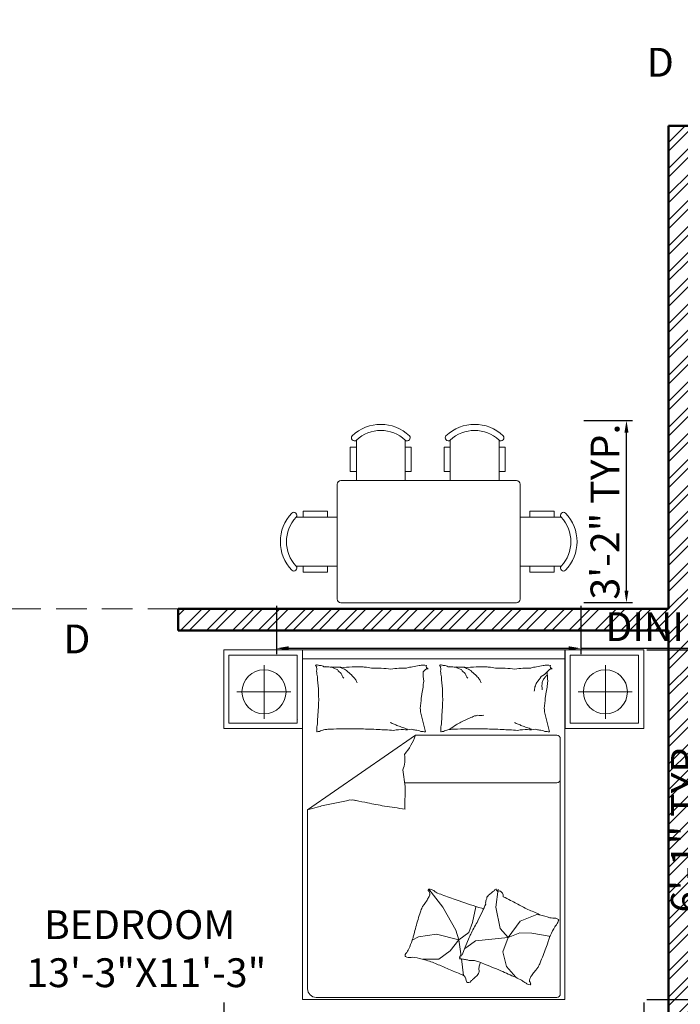
# Model space of a CAD drawing. Units: millimetres. Extents: x 67033 to 68301, y 155969 to 157209.
# Tile 12 of 17: x 67633 to 67771, y 156689 to 156894. Entities that reach past the tile are written whole.
import ezdxf

# ---------------------------------------------------------------- set-up
doc = ezdxf.new("R2010")
doc.units = ezdxf.units.MM
doc.linetypes.add('HIDDEN', pattern=[9.525, 6.35, -3.175])
for name, color, linetype, lineweight in [('A-ANNO-DIMS', 2, 'Continuous', 18), ('A-ANNO-TEXT', 7, 'Continuous', 18), ('A-AREA-IDEN', 3, 'Continuous', 18), ('A-FLOR-OVHD', 1, 'HIDDEN', 18), ('A-FLOR-PATT', 252, 'Continuous', 13), ('A-FURN', 8, 'Continuous', 18), ('A-WALL', 7, 'Continuous', 50), ('A-WALL-PATT', 8, 'Continuous', 13)]:
    doc.layers.add(name, color=color, linetype=linetype, lineweight=lineweight)
doc.styles.add('DIM_FONT', font='SIMPLEX.shx', dxfattribs={"width": 0.8})
doc.styles.get("Standard").update_dxf_attribs({"font": 'arial.ttf'})
doc.dimstyles.new('ISO-25', dxfattribs={"dimtxt": 6, "dimasz": 2.5, "dimexe": 1.25, "dimexo": 0.625, "dimtad": 1, "dimdec": 0, "dimlunit": 3, "dimtxsty": 'Standard', "dimcen": 2.5, "dimadec": 0, "dimazin": 0, "dimtfac": 1, "dimtdec": 0, "dimtmove": 0, "dimatfit": 3, "dimfxl": 1, "dimarcsym": 0})

# ---------------------------------------------------------------- blocks, each defined once
blk = doc.blocks.new('A$C79766A75')
for p, q in [((0.45, 1.9999), (0, 1.9999)), ((0, 1.9999), (0, 1.5499)), ((0.45, 1.5499), (0.45, 1.9999)), ((1.9506, 2), (0.4506, 2)), ((0.4506, 2), (0.4506, 0)), ((1.9506, 0), (1.9506, 2)), ((2.402, 1.9999), (1.952, 1.9999)), ((1.952, 1.9999), (1.952, 1.5499)), ((2.402, 1.5499), (2.402, 1.9999)), ((0.42, 1.9699), (0.03, 1.9699)), ((0.03, 1.9699), (0.03, 1.5799)), ((0.42, 1.5799), (0.42, 1.9699)), ((1.9506, 1.9476), (0.4506, 1.9476)), ((2.372, 1.9699), (1.982, 1.9699)), ((1.982, 1.9699), (1.982, 1.5799)), ((2.372, 1.5799), (2.372, 1.9699)), ((0.2304, 1.9125), (0.2304, 1.6061)), ((2.1824, 1.9125), (2.1824, 1.6061)), ((0.0743, 1.7595), (0.3834, 1.7595)), ((2.0263, 1.7595), (2.3354, 1.7595)), ((1.1461, 1.5617), (1.1254, 1.6443)), ((1.8553, 1.5617), (1.8346, 1.6443)), ((0.03, 1.5799), (0.42, 1.5799)), ((0.4234, 1.6034), (0.4228, 1.6034)), ((1.982, 1.5799), (2.372, 1.5799)), ((0, 1.5499), (0.45, 1.5499)), ((1.1536, 1.5317), (1.1461, 1.5617)), ((1.8628, 1.5317), (1.8553, 1.5617)), ((1.952, 1.5499), (2.402, 1.5499)), ((1.0972, 1.5115), (0.4791, 1.0841)), ((1.0972, 1.5115), (1.9048, 1.5115)), ((1.9248, 1.4915), (1.9248, 0.0322)), ((1.0383, 1.2184), (1.0246, 1.3138)), ((1.9048, 1.2389), (1.0354, 1.2389)), ((1.0365, 1.0883), (1.0383, 1.2184)), ((0.4791, 0.0622), (0.4791, 1.0841)), ((1.1731, 0.6316), (1.2523, 0.5276)), ((1.5696, 0.6317), (1.5559, 0.5286)), ((1.2523, 0.5276), (1.3274, 0.3973)), ((1.4223, 0.4407), (1.442, 0.5296)), ((1.5559, 0.5286), (1.5817, 0.4065)), ((1.6952, 0.4478), (1.7898, 0.4856)), ((1.7898, 0.4856), (1.8139, 0.4822)), ((1.3274, 0.3973), (1.3452, 0.342)), ((1.4025, 0.3834), (1.4223, 0.4407)), ((1.5817, 0.4065), (1.6264, 0.355)), ((1.6264, 0.355), (1.6952, 0.4478)), ((1.1139, 0.3597), (1.0779, 0.3397)), ((1.2167, 0.3736), (1.1139, 0.3597)), ((1.3452, 0.342), (1.2167, 0.3736)), ((1.2957, 0.2787), (1.3452, 0.342)), ((1.3452, 0.342), (1.4025, 0.3834)), ((1.3452, 0.342), (1.3569, 0.2478)), ((1.4034, 0.3558), (1.3803, 0.2995)), ((1.6264, 0.355), (1.4406, 0.3361)), ((1.5954, 0.2725), (1.6264, 0.355)), ((1.6264, 0.355), (1.6935, 0.3825)), ((1.6935, 0.3825), (1.7623, 0.379)), ((1.7623, 0.379), (1.8603, 0.3619)), ((1.8603, 0.3619), (1.8636, 0.3554)), ((1.3803, 0.2995), (1.3626, 0.256)), ((1.3907, 0.3), (1.3787, 0.2914)), ((1.4406, 0.3361), (1.3907, 0.3)), ((1.1376, 0.2313), (1.2305, 0.2313)), ((1.2305, 0.2313), (1.2957, 0.2787)), ((1.3588, 0.2331), (1.3706, 0.1385)), ((1.6161, 0.19), (1.5954, 0.2725)), ((1.6697, 0.1274), (1.6161, 0.19)), ((1.9048, 0.0122), (0.5291, 0.0122)), ((0.4506, 0), (1.9506, 0))]:
    blk.add_line(p, q)
for centre in [(0.2304, 1.7595), (2.1824, 1.7595)]:
    blk.add_circle(centre, 0.126)
for centre, radius, start, end in [((0.5246, 1.9378), 0.0251, 274.3025, 291.7883), ((0.5486, 1.9393), 0.0289, 239.3487, 274.3025), ((1.2338, 1.9378), 0.0251, 274.3025, 291.7883), ((1.2578, 1.9393), 0.0289, 239.3487, 274.3025), ((0.5232, 1.9139), 0.00342, 291.7883, 340.436), ((0.525, 1.9085), 0.00232, 340.436, 101.8931), ((0.5311, 1.9093), 0.00428, 201.9904, 281.8931), ((0.4996, 1.8889), 0.0328, 338.579, 8.1335), ((0.2896, 1.8253), 0.246, 8.1335, 12.1095), ((0.5465, 1.8994), 0.0156, 158.579, 201.9904), ((0.7297, 1.8867), 0.1983, 187.6809, 192.1095), ((0.5458, 1.8568), 0.0539, 59.3487, 84.7408), ((0.546, 1.0829), 0.8208, 84.7408, 88.0921), ((0.6118, 2.0005), 0.0992, 254.0648, 274.2159), ((0.6775, 1.9817), 0.0992, 233.9136, 254.0648), ((0.6362, 0.406), 1.4943, 88.0921, 90.5757), ((0.7304, 1.9449), 0.0992, 216.1766, 233.9136), ((0.7737, 2.1075), 0.234, 242.7604, 249.1397), ((0.7661, 1.8961), 0.0992, 198.4397, 216.1766), ((0.7591, 1.0293), 0.8732, 90.5757, 94.8018), ((0.738, 1.949), 0.0768, 231.6114, 242.7604), ((0.974, 2.1633), 0.3916, 226.1885, 231.6114), ((0.7631, 2.1919), 0.2897, 267.4614, 274.8018), ((0.8143, 2.0532), 0.1524, 259.8101, 267.4614), ((0.7515, 1.3747), 0.5293, 79.8101, 83.9133), ((0.8451, 0.8466), 1.049, 83.9133, 90), ((1.046, 1.2129), 0.6827, 90, 97.5469), ((1.1117, 1.6625), 0.2422, 97.5469, 105.744), ((1.0352, 2.2041), 0.3048, 278.4372, 285.744), ((1.1179, 2.0719), 0.1611, 270, 278.4372), ((1.171, 1.8579), 0.0342, 94.4002, 153.4195), ((1.6324, 1.8735), 0.4918, 180, 186.2324), ((1.1592, 2.0011), 0.0904, 258.7276, 270), ((1.1709, 1.9049), 0.0131, 153.4195, 258.7276), ((1.2325, 1.9139), 0.00342, 291.7883, 340.436), ((1.2342, 1.9085), 0.00232, 340.436, 101.8931), ((1.2404, 1.9093), 0.00428, 201.9904, 281.8931), ((1.2088, 1.8889), 0.0328, 338.579, 8.1335), ((0.9988, 1.8253), 0.246, 8.1335, 12.1095), ((1.2558, 1.8994), 0.0156, 158.579, 201.9904), ((1.4389, 1.8867), 0.1983, 187.6809, 192.1095), ((1.2551, 1.8568), 0.0539, 59.3487, 84.7408), ((1.2552, 1.0829), 0.8208, 84.7408, 88.0921), ((1.3211, 2.0005), 0.0992, 254.0648, 274.2159), ((1.3868, 1.9817), 0.0992, 233.9136, 254.0648), ((1.3455, 0.406), 1.4943, 88.0921, 90.5757), ((1.4396, 1.9449), 0.0992, 216.1766, 233.9136), ((1.4829, 2.1075), 0.234, 242.7604, 249.1397), ((1.4753, 1.8961), 0.0992, 198.4397, 216.1766), ((1.4683, 1.0293), 0.8732, 90.5757, 94.8018), ((1.4473, 1.949), 0.0768, 231.6114, 242.7604), ((1.6833, 2.1633), 0.3916, 226.1885, 231.6114), ((1.4724, 2.1919), 0.2897, 267.4614, 274.8018), ((1.5236, 2.0532), 0.1524, 259.8101, 267.4614), ((1.4607, 1.3747), 0.5293, 79.8101, 83.9133), ((1.5543, 0.8466), 1.049, 83.9133, 90), ((1.7552, 1.2129), 0.6827, 90, 97.5469), ((1.821, 1.6625), 0.2422, 97.5469, 105.744), ((1.7444, 2.2041), 0.3048, 278.4372, 285.744), ((1.7511, 1.9723), 0.1399, 297.2036, 314.9024), ((1.8271, 2.0719), 0.1611, 270, 278.4372), ((1.8802, 1.8579), 0.0342, 94.4002, 153.4195), ((2.3416, 1.8735), 0.4918, 180, 186.2324), ((1.8684, 2.0011), 0.0904, 258.7276, 270), ((1.8802, 1.9049), 0.0131, 153.4195, 258.7276), ((1.4472, 1.8987), 0.9131, 183.3687, 187.6809), ((0.9057, 1.9982), 0.2252, 219.0349, 226.1885), ((0.7932, 1.8591), 0.0493, 208.3168, 219.0349), ((0.9392, 1.9062), 0.2002, 203.0028, 208.3168), ((1.3446, 1.7858), 0.204, 170.3156, 180), ((2.1565, 1.8987), 0.9131, 183.3687, 187.6809), ((1.615, 1.9982), 0.2252, 219.0349, 226.1885), ((1.5025, 1.8591), 0.0493, 208.3168, 219.0349), ((1.6484, 1.9062), 0.2002, 203.0028, 208.3168), ((1.6554, 1.8529), 0.1399, 332.6012, 343.485), ((1.6908, 1.9123), 0.1399, 314.9024, 332.6012), ((1.7653, 1.8132), 0.0562, 341.2201, 0), ((1.6307, 1.8895), 0.2056, 338.1851, 341.2201), ((1.6887, 1.8881), 0.1511, 334.6449, 338.1851), ((1.7896, 1.8667), 0.0526, 318.5571, 334.6449), ((1.784, 1.9167), 0.0899, 306.2641, 318.5571), ((2.0538, 1.7858), 0.204, 170.3156, 180), ((1.2208, 1.7573), 0.6787, 178.3669, 183.3687), ((0.8192, 1.792), 0.3171, 347.8016, 351.9949), ((2.0027, 1.5994), 0.882, 167.8016, 170.3156), ((1.9301, 1.7573), 0.6787, 178.3669, 183.3687), ((1.6404, 1.8023), 0.1399, 343.485, 354.3689), ((1.73, 1.7719), 0.0915, 0, 14.6851), ((1.5284, 1.792), 0.3171, 347.8016, 351.9949), ((2.7119, 1.5994), 0.882, 167.8016, 170.3156), ((1.9066, 1.6447), 1.3652, 176.945, 178.3669), ((0.4711, 1.7556), 0.6588, 351.9949, 357.3351), ((2.6158, 1.6447), 1.3652, 176.945, 178.3669), ((1.1803, 1.7556), 0.6588, 351.9949, 357.3351), ((14.1519, 0.85), 13.6356, 176.49514, 176.94504), ((1.0578, 1.6474), 0.0677, 357.3351, 14.0452), ((14.8612, 0.85), 13.6356, 176.49514, 176.94504), ((1.767, 1.6474), 0.0677, 357.3351, 14.0452), ((0.8521, 1.5209), 0.3212, 170.0016, 176.4951), ((0.6583, 0.9067), 0.7387, 64.6889, 66.5156), ((1.5613, 1.5209), 0.3212, 170.0016, 176.4951), ((1.1895, 1.8508), 0.3126, 296.4985, 302.135), ((0.7658, 2.8912), 1.4323, 294.3265, 296.4985), ((1.226, 2.0834), 0.5066, 290.6743, 294.3265), ((1.4305, 1.6796), 0.058, 274.0828, 290.6743), ((1.4679, 1.8969), 0.2721, 266.4448, 274.0828), ((1.3675, 0.9067), 0.7387, 64.6889, 66.5156), ((0.513, 1.535), 0.0193, 350.0016, 16.6978), ((0.5322, 1.5304), 0.00132, 16.6978, 97.1204), ((0.5579, 1.4467), 0.0875, 97.1204, 106.2212), ((0.5822, 1.4654), 0.0767, 106.2212, 117.2841), ((0.5507, 1.5832), 0.0453, 282.869, 297.2841), ((0.5623, 1.6885), 0.1459, 273.574, 282.869), ((0.589, 2.7103), 1.164, 270.2865, 273.574), ((0.7584, 7.2662), 5.7185, 269.0296, 270.2865), ((0.9401, 4.9065), 3.3622, 267.3904, 269.0296), ((0.9811, 2.7573), 1.2165, 265.3824, 267.3904), ((0.8583, 0.139), 1.4048, 85.3824, 87.2509), ((1.0175, 1.3138), 0.2301, 87.2509, 101.5586), ((0.7015, 0.888), 0.7387, 66.5156, 68.3423), ((0.7501, 0.8688), 0.7387, 68.3423, 70.572), ((0.8043, 0.8497), 0.7387, 70.572, 72.8018), ((1.0449, 1.6886), 0.1459, 263.5659, 281.5586), ((1.1099, 1.6599), 0.1197, 252.6136, 263.5659), ((1.0587, 1.3144), 0.2297, 72.6136, 80.5159), ((1.108, 1.2635), 0.2708, 80.5159, 85.9171), ((1.1535, 1.5308), 0.000917, 85.9171, 194.0449), ((1.2222, 1.535), 0.0193, 350.0016, 16.6978), ((1.2414, 1.5304), 0.00132, 16.6978, 97.1204), ((1.2671, 1.4467), 0.0875, 97.1204, 106.2212), ((1.2914, 1.4654), 0.0767, 106.2212, 117.2841), ((1.2599, 1.5832), 0.0453, 282.869, 297.2841), ((1.2716, 1.6885), 0.1459, 273.574, 282.869), ((0.9025, 2.1618), 0.7286, 302.135, 305.8263), ((1.2982, 2.7103), 1.164, 270.2865, 273.574), ((1.4677, 7.2662), 5.7185, 269.0296, 270.2865), ((1.6493, 4.9065), 3.3622, 267.3904, 269.0296), ((1.6903, 2.7573), 1.2165, 265.3824, 267.3904), ((1.5676, 0.139), 1.4048, 85.3824, 87.2509), ((1.7268, 1.3138), 0.2301, 87.2509, 101.5586), ((1.4107, 0.888), 0.7387, 66.5156, 68.3423), ((1.4594, 0.8688), 0.7387, 68.3423, 70.572), ((1.5136, 0.8497), 0.7387, 70.572, 72.8018), ((1.7541, 1.6886), 0.1459, 263.5659, 281.5586), ((1.8192, 1.6599), 0.1197, 252.6136, 263.5659), ((1.7679, 1.3144), 0.2297, 72.6136, 80.5159), ((1.8172, 1.2635), 0.2708, 80.5159, 85.9171), ((1.8627, 1.5308), 0.000917, 85.9171, 194.0449), ((0.745, 1.6407), 0.3751, 320.3555, 339.8512), ((1.9048, 1.4915), 0.02, 0, 90), ((0.8556, 1.3759), 0.1801, 339.8512, 8.1356), ((1.9048, 1.2589), 0.02, 270, 0), ((-0.1888, 5.1029), 4.0646, 280.7276, 282.9255), ((0.7282, 1.1989), 0.0581, 262.2696, 280.7276), ((0.7833, 1.3309), 0.1942, 256.8096, 262.2696), ((0.2481, -1.3253), 2.5158, 76.8096, 78.3259), ((-0.0248, 2.8487), 1.8351, 285.9352, 287.7364), ((0.3872, 1.7415), 0.6574, 282.9255, 285.9352), ((0.3953, -1.4284), 2.588, 78.3259, 80.505), ((0.413, -2.64), 3.7801, 80.505, 82.308), ((1.1752, 0.6267), 0.0063, 166.7192, 233.4208), ((1.1734, 0.6272), 0.00443, 93.9484, 166.7192), ((1.163, 0.6103), 0.0142, 10.4074, 53.4208), ((1.1755, 0.5964), 0.0352, 69.6548, 93.9484), ((1.1669, 0.5731), 0.0601, 51.4146, 69.6548), ((1.2538, 0.682), 0.0792, 231.4146, 247.2931), ((1.1426, 1.1456), 0.6605, 306.2163, 307.2151), ((1.7751, 0.3162), 0.3825, 126.2163, 127.5287), ((1.5806, 0.5924), 0.0452, 127.5287, 134.1274), ((1.5093, 0.6825), 0.0697, 308.8136, 314.1274), ((1.5706, 0.6318), 0.0127, 176.7545, 308.8136), ((1.5621, 0.59), 0.0359, 356.7545, 62.7098), ((0.9961, 0.6678), 0.194, 320.2995, 329.0944), ((0.8605, 0.749), 0.352, 329.0944, 333.1821), ((1.1396, 0.6079), 0.0393, 333.1821, 345.4291), ((1.1011, 0.5989), 0.0771, 2.7286, 10.4074), ((1.1628, 0.6019), 0.0153, 345.4291, 2.7286), ((1.5463, 1.3811), 0.8371, 247.2931, 249.8713), ((3.0113, 5.3783), 5.0942, 249.8713, 250.9164), ((2.374, 3.5362), 3.145, 250.9164, 253.3915), ((1.5435, 0.5526), 0.0458, 157.5838, 188.0492), ((1.4828, 0.5833), 0.0226, 324.1064, 8.0492), ((1.4519, 0.6426), 0.0774, 313.5224, 324.1064), ((1.383, 0.7705), 0.2176, 307.2151, 313.5224), ((0.2201, -2.1858), 3.0972, 62.7098, 63.5853), ((2.5711, 2.3551), 2.0162, 242.5001, 243.5853), ((1.3115, 0.4414), 0.1965, 153.9265, 162.1604), ((1.2077, 0.4922), 0.081, 140.2995, 153.9265), ((1.5084, 0.6341), 0.1166, 253.3915, 259.2634), ((2.4089, 0.1204), 1.0054, 154.9471, 157.5838), ((4.5245, 5.9445), 6.1019, 242.15178, 242.50014), ((-0.9881, -4.647), 5.8383, 62.15178, 62.50792), ((1.5182, -0.068), 0.6236, 62.5079, 69.2514), ((3.0311, -0.112), 2.003, 162.1604, 164.7375), ((2.9813, -0.2643), 1.6868, 152.9116, 154.9471), ((1.7121, 0.0657), 0.43, 69.2514, 77.3748), ((1.8682, 0.4049), 0.063, 77.3748, 93.3881), ((1.8955, 0.5247), 0.0599, 256.9598, 273.3881), ((1.9257, 0.5082), 0.0509, 238.3083, 256.9598), ((1.9279, 0.441), 0.0168, 130.5086, 180.9614), ((1.9201, 0.4587), 0.0058, 180.9614, 238.3083), ((2.6887, -0.0186), 1.6481, 164.7375, 166.159), ((2.8096, -0.3311), 1.5652, 150.064, 152.9116), ((-0.5166, 1.5491), 2.6619, 333.6668, 334.8268), ((1.8435, 0.4743), 0.0755, 310.5086, 333.6668), ((-1.4109, 1.284), 2.6619, 338.0627, 339.2227), ((0.9098, 0.4035), 0.1798, 339.2227, 343.6878), ((0.5589, 0.5062), 0.5454, 343.6878, 346.159), ((1.2176, 0.4627), 0.2143, 330.064, 337.7645), ((1.3456, 0.5261), 0.5454, 339.2919, 341.7631), ((1.701, 0.4319), 0.1798, 334.8268, 339.2919), ((0.9882, 0.3177), 0.0755, 314.9045, 338.0627), ((3.6966, -0.4634), 2.003, 157.7645, 160.3416), ((3.4079, -0.2212), 1.6481, 160.3416, 161.7631), ((1.0533, 0.2524), 0.0168, 134.9045, 185.3572), ((1.0424, 0.2513), 0.0058, 185.3572, 242.7041), ((1.0631, 0.2914), 0.0509, 242.7041, 261.3557), ((1.0645, 0.3003), 0.0599, 261.3557, 277.784), ((1.0811, 0.1786), 0.063, 81.7707, 97.784), ((1.0286, -0.1846), 0.43, 73.6473, 81.7707), ((0.974, -0.3705), 0.6236, 66.9038, 73.6473), ((1.3465, 0.2383), 0.00467, 287.1867, 70.6201), ((1.3486, 0.2247), 0.0092, 70.6201, 94.2593), ((1.3694, 0.234), 0.0231, 107.1867, 157.7645), ((1.3563, 0.267), 0.034, 262.0178, 274.2593), ((1.4091, 0.4221), 0.1955, 255.1193, 262.0178), ((1.358, 0.0507), 0.1794, 75.1193, 82.3216), ((-1.0716, -5.1672), 5.8383, 66.54766, 66.9038), ((3.6805, 5.7866), 6.1019, 246.54766, 246.89602), ((2.0773, 2.0287), 2.0162, 246.896, 247.9812), ((1.4096, 0.153), 0.0712, 82.3216, 94.5118), ((1.4285, 0.2893), 0.0663, 261.8784, 274.5118), ((1.4755, 0.332), 0.1166, 248.9957, 261.8784), ((2.7121, 3.1012), 3.145, 246.5205, 248.9957), ((1.505, 0.1766), 0.0458, 161.9797, 192.4451), ((2.4175, -0.1202), 1.0054, 160.6552, 161.9797), ((1.6279, 0.2819), 0.194, 315.9036, 324.6985), ((1.856, 0.1288), 0.081, 135.9036, 149.5306), ((1.9797, 0.1108), 0.1965, 149.5306, 157.7645), ((0.1602, -2.7118), 3.0972, 67.1056, 67.9812), ((1.3512, 0.1084), 0.0359, 1.1504, 67.1056), ((1.6722, -0.1762), 0.3825, 130.6122, 131.9246), ((0.9933, 0.6156), 0.6605, 310.6122, 311.611), ((1.2874, 0.2845), 0.2176, 311.611, 317.9183), ((1.3914, 0.1905), 0.0774, 317.9183, 328.5023), ((1.4382, 0.1619), 0.0226, 328.5023, 12.4451), ((3.6993, 4.7998), 5.0942, 245.4754, 246.5205), ((2.051, 0.8725), 0.8371, 242.8972, 245.4754), ((1.7345, 0.1188), 0.0153, 341.0332, 358.3327), ((1.6723, 0.1058), 0.0771, 358.3327, 6.0115), ((1.7162, 0.1388), 0.0393, 328.7862, 341.0332), ((1.4661, 0.3294), 0.352, 324.6985, 328.7862), ((0.5291, 0.0622), 0.05, 180, 270), ((1.3997, 0.1094), 0.0127, 181.1504, 313.2095), ((1.3607, 0.1509), 0.0697, 313.2095, 318.5233), ((1.4468, 0.0748), 0.0452, 131.9246, 138.5233), ((1.7576, 0.1689), 0.0792, 227.0187, 242.8972), ((1.6963, 0.0438), 0.0601, 47.0187, 65.2589), ((1.737, 0.0526), 0.0352, 65.2589, 89.5525), ((1.7401, 0.0928), 0.0142, 6.0115, 49.0249), ((1.756, 0.0832), 0.00443, 89.5525, 162.3233), ((1.7602, 0.0924), 0.0063, 162.3233, 229.0249), ((1.9048, 0.0322), 0.02, 270, 0)]:
    blk.add_arc(centre, radius, start, end)
at = {"style": 'DIM_FONT', "text_generation_flag": 4, "width": 0.8, "flags": 9}
for tag in ['XSIZE', 'YSIZE']:
    blk.add_attdef(tag, (1.9506, 2), '', height=0.0005, rotation=180, dxfattribs=at)
blk = doc.blocks.new('table dining')
for p, q in [((67480.1, 156784.21), (67480.1, 156775.8)), ((67490.26, 156775.8), (67490.26, 156784.21)), ((67499.62, 156784.21), (67499.62, 156775.8)), ((67509.78, 156775.8), (67509.78, 156784.21)), ((67480.1, 156782.75), (67478.83, 156782.75)), ((67478.83, 156777.67), (67478.83, 156782.75)), ((67490.26, 156782.75), (67491.53, 156782.75)), ((67491.53, 156777.67), (67491.53, 156782.75)), ((67499.62, 156782.75), (67498.35, 156782.75)), ((67498.35, 156777.67), (67498.35, 156782.75)), ((67509.78, 156782.75), (67511.05, 156782.75)), ((67511.05, 156777.67), (67511.05, 156782.75)), ((67476.85, 156775.8), (67513.43, 156775.8)), ((67480.1, 156777.67), (67478.83, 156777.67)), ((67490.26, 156777.67), (67491.53, 156777.67)), ((67499.62, 156777.67), (67498.35, 156777.67)), ((67509.78, 156777.67), (67511.05, 156777.67)), ((67476.09, 156751.17), (67476.09, 156775.04)), ((67514.19, 156751.17), (67514.19, 156775.04)), ((67476.09, 156768.18), (67467.57, 156768.18)), ((67469.03, 156768.18), (67469.03, 156769.45)), ((67474.11, 156769.45), (67469.03, 156769.45)), ((67474.11, 156768.18), (67474.11, 156769.45)), ((67514.19, 156768.18), (67522.71, 156768.18)), ((67516.16, 156768.18), (67516.16, 156769.45)), ((67516.16, 156769.45), (67521.24, 156769.45)), ((67521.24, 156768.18), (67521.24, 156769.45)), ((67467.57, 156758.02), (67476.09, 156758.02)), ((67469.03, 156758.02), (67469.03, 156756.75)), ((67474.11, 156758.02), (67474.11, 156756.75)), ((67522.71, 156758.02), (67514.19, 156758.02)), ((67516.16, 156758.02), (67516.16, 156756.75)), ((67521.24, 156758.02), (67521.24, 156756.75)), ((67474.11, 156756.75), (67469.03, 156756.75)), ((67516.16, 156756.75), (67521.24, 156756.75)), ((67476.85, 156750.4), (67513.43, 156750.4))]:
    blk.add_line(p, q)
for centre, radius, start, end in [((67485.18, 156778.87), 8.64, 46.4394, 133.5606), ((67485.18, 156778.87), 7.37, 46.4394, 133.5606), ((67504.7, 156778.87), 8.64, 46.4394, 133.5606), ((67504.7, 156778.87), 7.37, 46.4394, 133.5606), ((67479.7, 156784.71), 0.637, 138.3417, 308.7795), ((67490.66, 156784.71), 0.637, 231.2205, 41.6583), ((67499.22, 156784.71), 0.637, 138.3417, 308.7795), ((67510.18, 156784.71), 0.637, 231.2205, 41.6583), ((67476.85, 156775.04), 0.762, 90, 180), ((67513.43, 156775.04), 0.762, 0, 90), ((67472.91, 156763.1), 8.64, 136.4394, 223.5606), ((67472.91, 156763.1), 7.37, 136.4394, 223.5606), ((67467.07, 156768.58), 0.637, 321.2205, 131.6583), ((67523.2, 156768.58), 0.637, 48.3417, 218.7795), ((67517.37, 156763.1), 7.37, 316.4394, 43.5606), ((67517.37, 156763.1), 8.64, 316.4394, 43.5606), ((67467.07, 156757.62), 0.637, 228.3417, 38.7795), ((67523.2, 156757.62), 0.637, 141.2205, 311.6583), ((67476.85, 156751.17), 0.762, 180, 270), ((67513.43, 156751.17), 0.762, 270, 0)]:
    blk.add_arc(centre, radius, start, end)
blk = doc.blocks.new('*D57')
at = {"layer": 'A-ANNO-DIMS', "color": 0, "lineweight": -2, "transparency": 16777216}
for p, q in [((67675.78, 156689.05), (67675.78, 156675.31)), ((67763.19, 156689.05), (67763.19, 156675.31)), ((67678.28, 156676.56), (67760.69, 156676.56)), ((67763.19, 156676.56), (67873.56, 156676.56))]:
    blk.add_line(p, q, dxfattribs=at)
at = {"layer": 'A-ANNO-DIMS', "color": 0, "transparency": 16777216}
for points in [[(67678.28, 156676.98), (67678.28, 156676.14), (67675.78, 156676.56)], [(67760.69, 156676.98), (67760.69, 156676.14), (67763.19, 156676.56)]]:
    blk.add_solid(points, dxfattribs=at)
at = {"layer": 'Defpoints', "color": 0, "transparency": 16777216}
for p in [(67675.78, 156689.67), (67763.19, 156689.67), (67763.19, 156676.56)]:
    blk.add_point(p, dxfattribs=at)
at = {"layer": 'A-ANNO-DIMS', "color": 0, "transparency": 16777216, "insert": (67819.62, 156680.29), "char_height": 6, "attachment_point": 5}
blk.add_mtext('DOUBLE BED 7\'-3 1/2" TYP.', dxfattribs=at)
blk = doc.blocks.new('*D58')
at = {"layer": 'A-ANNO-DIMS', "color": 0, "lineweight": -2, "transparency": 16777216}
for p, q in [((67763.82, 156762.48), (67777.55, 156762.48)), ((67776.3, 156692.17), (67776.3, 156759.98)), ((67763.82, 156689.67), (67777.55, 156689.67))]:
    blk.add_line(p, q, dxfattribs=at)
at = {"layer": 'A-ANNO-DIMS', "color": 0, "transparency": 16777216}
for points in [[(67775.89, 156759.98), (67776.72, 156759.98), (67776.3, 156762.48)], [(67775.89, 156692.17), (67776.72, 156692.17), (67776.3, 156689.67)]]:
    blk.add_solid(points, dxfattribs=at)
at = {"layer": 'Defpoints', "color": 0, "transparency": 16777216}
for p in [(67763.19, 156762.48), (67776.3, 156762.48), (67763.19, 156689.67)]:
    blk.add_point(p, dxfattribs=at)
at = {"layer": 'A-ANNO-DIMS', "color": 0, "transparency": 16777216, "insert": (67772.62, 156726.07), "char_height": 6, "attachment_point": 5, "rotation": 90}
blk.add_mtext('6\'-1" TYP.', dxfattribs=at)
blk = doc.blocks.new('*D67')
at = {"layer": 'A-ANNO-DIMS', "color": 0, "lineweight": -2, "transparency": 16777216}
for p, q in [((67686.77, 156771.63), (67686.77, 156761.51)), ((67750.09, 156771.63), (67750.09, 156761.51)), ((67689.27, 156762.76), (67747.59, 156762.76)), ((67750.09, 156762.76), (67864.65, 156762.76))]:
    blk.add_line(p, q, dxfattribs=at)
at = {"layer": 'A-ANNO-DIMS', "color": 0, "transparency": 16777216}
for points in [[(67689.27, 156763.18), (67689.27, 156762.34), (67686.77, 156762.76)], [(67747.59, 156763.18), (67747.59, 156762.34), (67750.09, 156762.76)]]:
    blk.add_solid(points, dxfattribs=at)
at = {"layer": 'Defpoints', "color": 0, "transparency": 16777216}
for p in [(67686.77, 156772.26), (67750.09, 156772.26), (67750.09, 156762.76)]:
    blk.add_point(p, dxfattribs=at)
at = {"layer": 'A-ANNO-DIMS', "color": 0, "transparency": 16777216, "insert": (67808.62, 156766.49), "char_height": 6, "attachment_point": 5}
blk.add_mtext('DINING TABLE 5\'-3 1/2" TYP.', dxfattribs=at)
blk = doc.blocks.new('*D68')
at = {"layer": 'A-ANNO-DIMS', "color": 0, "lineweight": -2, "transparency": 16777216}
for p, q in [((67750.72, 156810.16), (67760.84, 156810.16)), ((67759.59, 156774.76), (67759.59, 156807.66)), ((67750.72, 156772.26), (67760.84, 156772.26))]:
    blk.add_line(p, q, dxfattribs=at)
at = {"layer": 'A-ANNO-DIMS', "color": 0, "transparency": 16777216}
for points in [[(67759.18, 156807.66), (67760.01, 156807.66), (67759.59, 156810.16)], [(67759.18, 156774.76), (67760.01, 156774.76), (67759.59, 156772.26)]]:
    blk.add_solid(points, dxfattribs=at)
at = {"layer": 'Defpoints', "color": 0, "transparency": 16777216}
for p in [(67750.09, 156810.16), (67759.59, 156810.16), (67750.09, 156772.26)]:
    blk.add_point(p, dxfattribs=at)
at = {"layer": 'A-ANNO-DIMS', "color": 0, "transparency": 16777216, "insert": (67755.9, 156791.21), "char_height": 6, "attachment_point": 5, "rotation": 90}
blk.add_mtext('3\'-2" TYP.', dxfattribs=at)
blk = doc.blocks.new('*D112')
at = {"layer": 'A-ANNO-DIMS', "color": 0, "lineweight": -2, "transparency": 16777216}
for p, q in [((67601.44, 157144.49), (67868.32, 157144.49)), ((67867.07, 157141.99), (67867.07, 156564.99)), ((67768.94, 156562.49), (67868.32, 156562.49))]:
    blk.add_line(p, q, dxfattribs=at)
at = {"layer": 'A-ANNO-DIMS', "color": 0, "transparency": 16777216}
for points in [[(67866.65, 157141.99), (67867.48, 157141.99), (67867.07, 157144.49)], [(67866.65, 156564.99), (67867.48, 156564.99), (67867.07, 156562.49)]]:
    blk.add_solid(points, dxfattribs=at)
at = {"layer": 'Defpoints', "color": 0, "transparency": 16777216}
for p in [(67600.82, 157144.49), (67768.32, 156562.49), (67867.07, 156562.49)]:
    blk.add_point(p, dxfattribs=at)
at = {"layer": 'A-ANNO-DIMS', "color": 0, "transparency": 16777216, "insert": (67863.38, 156853.49), "char_height": 6, "attachment_point": 5, "rotation": 90}
blk.add_mtext('48\'-6"', dxfattribs=at)

msp = doc.modelspace()

# ---------------------------------------------------------------- hatches: boundary and pattern name
at = {"layer": 'A-FLOR-PATT'}
h = msp.add_hatch(dxfattribs=at)
h.set_pattern_fill('NET', color=256, scale=2.1)
h.set_pattern_definition([(0, (429.8785, 0), (0, 6.6675), []), (90, (429.8785, 0), (-6.6675, 4e-16), [])])
h.paths.add_polyline_path([(67823.43, 156741.13), (67824.62, 156742.23), (67832.57, 156742.26), (67832.57, 156731.79), (67832.57, 156721.36), (67824.62, 156721.36), (67823.54, 156722.36), (67809.23, 156724.15), (67807.41, 156724.7), (67805.06, 156726.38), (67803.4, 156728.81), (67802.63, 156731.7), (67803.17, 156734.03), (67804.67, 156736.58), (67806.89, 156738.43), (67809.3, 156739.26)], flags=16)
h.paths.add_polyline_path([(67759.9, 156741.43), (67815.84, 156741.43), (67815.84, 156763.82), (67759.9, 156763.82)], flags=9)
at = {"layer": 'A-WALL-PATT'}
h = msp.add_hatch(dxfattribs=at)
h.set_pattern_fill('ANSI32', color=256, scale=0.4)
h.set_pattern_definition([(45, (429.8785, 0), (-2.69407684, 2.69407684), []), (45, (431.6745, 0), (-2.69407684, 2.69407684), [])])
h.paths.add_polyline_path([(67837.32, 156941.99), (67832.82, 156941.99), (67832.82, 156802.49), (67772.82, 156802.49), (67772.82, 156822.09), (67772.82, 156871.49), (67768.32, 156871.49), (67768.32, 156770.99), (67666.32, 156770.99), (67666.32, 156766.49), (67768.32, 156766.49), (67768.32, 156685.49), (67772.82, 156685.49), (67772.82, 156797.99), (67832.82, 156797.99), (67832.82, 156767.19), (67837.32, 156767.19)])

# ---------------------------------------------------------------- linework, layer by layer
at = {"layer": 'A-FLOR-OVHD'}
msp.add_line((67666.32, 156770.99), (67626.86, 156770.99), dxfattribs=at)
at = {"layer": 'A-WALL'}
for p, q in [((67768.32, 156871.49), (67768.32, 156770.99)), ((67768.32, 156871.49), (67772.82, 156871.49)), ((67666.32, 156770.99), (67666.32, 156766.49)), ((67666.32, 156770.99), (67768.32, 156770.99)), ((67666.32, 156766.49), (67768.32, 156766.49)), ((67768.32, 156766.49), (67768.32, 156685.49))]:
    msp.add_line(p, q, dxfattribs=at)

# ---------------------------------------------------------------- block references
at = {"layer": 'A-FURN'}
msp.add_blockref('table dining', (223.29, 21.85), dxfattribs=at)
at = {"layer": 'A-FURN', "xscale": 36.39326745080975, "yscale": 36.39326745080975, "zscale": 36.39326745080975}
msp.add_blockref('A$C79766A75', (67675.78, 156689.67), dxfattribs=at)

# ---------------------------------------------------------------- texts
at = {"layer": 'A-ANNO-TEXT', "char_height": 6, "attachment_point": 1}
for insert in [(67758.33, 156887.7), (67636.89, 156767.71)]:
    msp.add_mtext_dynamic_manual_height_columns('   D', width=19.5287, gutter_width=12.5, heights=[0], dxfattribs=dict(at, insert=insert))
at = {"layer": 'A-AREA-IDEN', "insert": (67634.69, 156708.26), "char_height": 6, "attachment_point": 1}
msp.add_mtext_dynamic_manual_height_columns('  BEDROOM \\P13\'-3"X11\'-3"', width=59.4046, gutter_width=12.5, heights=[0], dxfattribs=at)

# ---------------------------------------------------------------- dimensions: what is measured, and where the dimension line sits
at = {"layer": 'A-ANNO-DIMS'}
dim = msp.add_linear_dim(base=(67867.07, 156562.49), p1=(67600.82, 157144.49), p2=(67768.32, 156562.49), angle=90, dimstyle='ISO-25', override={"dimdec": 1, "dimlfac": 1, "dimrnd": 0, "dimzin": 1, "dimdsep": 46, "dimlunit": 4, "dimfrac": 2}, dxfattribs=at)
dim.commit()
dim.dimension.update_dxf_attribs({"geometry": '*D112', "text_midpoint": (67863.38, 156853.49)})
for base, p1, p2, picture, middle in [((67759.59, 156810.16), (67750.09, 156772.26), (67750.09, 156810.16), '*D68', (67755.9, 156791.21)), ((67776.3, 156762.48), (67763.19, 156689.67), (67763.19, 156762.48), '*D58', (67772.62, 156726.07))]:
    dim = msp.add_linear_dim(base=base, p1=p1, p2=p2, angle=90, text='<> TYP.', dimstyle='ISO-25', override={"dimdec": 1, "dimrnd": 0, "dimzin": 1, "dimlunit": 4, "dimfrac": 2}, dxfattribs=at)
    dim.commit()
    dim.dimension.update_dxf_attribs({"geometry": picture, "text_midpoint": middle})
for base, p1, p2, text, picture, middle in [((67750.09, 156762.76), (67686.77, 156772.26), (67750.09, 156772.26), 'DINING TABLE <> TYP.', '*D67', (67808.62, 156766.49)), ((67763.19, 156676.56), (67675.78, 156689.67), (67763.19, 156689.67), 'DOUBLE BED <> TYP.', '*D57', (67819.62, 156680.29))]:
    dim = msp.add_linear_dim(base=base, p1=p1, p2=p2, text=text, dimstyle='ISO-25', override={"dimdec": 1, "dimrnd": 0, "dimzin": 1, "dimlunit": 4, "dimfrac": 2}, dxfattribs=at)
    dim.commit()
    dim.dimension.update_dxf_attribs({"geometry": picture, "text_midpoint": middle})

doc.saveas('drawing.dxf')
